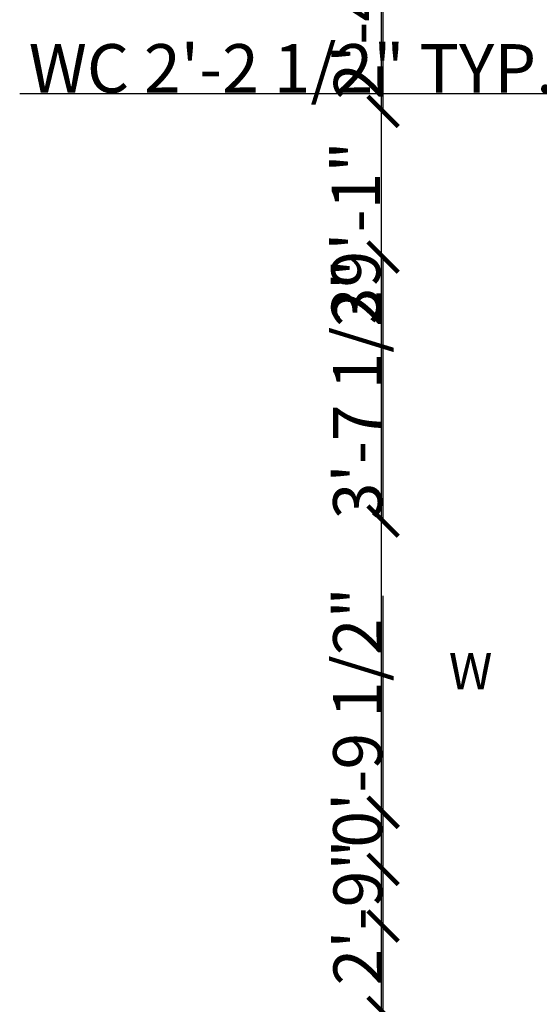
# Model space of a CAD drawing. Units: inches. Extents: x 2094 to 2639, y 1426 to 1997.
# Tile 2 of 8: x 2094 to 2180, y 1567 to 1730. Entities that reach past the tile are written whole.
import ezdxf

# ---------------------------------------------------------------- set-up
doc = ezdxf.new("R2010")
doc.units = ezdxf.units.IN
doc.layers.add('A-ANNO-DIMS', color=2, linetype='Continuous', lineweight=18)
doc.layers.add('A-ANNO-TEXT', color=7, linetype='Continuous', lineweight=18)
doc.styles.get("Standard").update_dxf_attribs({"font": 'arial.ttf'})
doc.dimstyles.get("Standard").update_dxf_attribs({"dimtxt": 8, "dimasz": 5, "dimexe": 0.18, "dimexo": 0.0625, "dimgap": 0.09, "dimtad": 1, "dimdec": 1, "dimzin": 0, "dimdsep": 46, "dimlunit": 4, "dimtxsty": 'Standard', "dimblk": 'ARCHTICK', "dimcen": 0.09, "dimse1": 1, "dimse2": 1, "dimadec": 0, "dimazin": 0, "dimtfac": 1, "dimtdec": 1, "dimtofl": 0, "dimtmove": 0, "dimatfit": 3, "dimfxl": 1, "dimtolj": 1, "dimtzin": 0, "dimarcsym": 0})

# ---------------------------------------------------------------- blocks, each defined once
blk = doc.blocks.new('_ArchTick')
at = {"color": 0, "linetype": 'ByBlock', "const_width": 0.15}
blk.add_lwpolyline([(-0.5, -0.5), (0.5, 0.5)], dxfattribs=at)
blk = doc.blocks.new('*D14')
at = {"layer": 'A-ANNO-DIMS', "color": 0, "lineweight": -2, "transparency": 16777216}
blk.add_line((2154, 1928.9), (2154, 1459.9), dxfattribs=at)
at = {"layer": 'Defpoints', "color": 0, "transparency": 16777216}
for p in [(2180.06, 1928.9), (2154, 1459.9), (2180.06, 1459.9)]:
    blk.add_point(p, dxfattribs=at)
at = {"layer": 'A-ANNO-DIMS', "color": 0, "lineweight": -2, "transparency": 16777216, "xscale": 5, "yscale": 5, "zscale": 5}
for p, rotation in [((2154, 1928.9), 90), ((2154, 1459.9), 270)]:
    blk.add_blockref('_ArchTick', p, dxfattribs=dict(at, rotation=rotation))
at = {"layer": 'A-ANNO-DIMS', "color": 0, "transparency": 16777216, "insert": (2149.82, 1694.4), "char_height": 8, "attachment_point": 5, "rotation": 90}
blk.add_mtext('\\A1;39\'-1"', dxfattribs=at)
blk = doc.blocks.new('*D39')
at = {"layer": 'A-ANNO-DIMS', "color": 0, "lineweight": -2, "transparency": 16777216}
for p, q in [((2189.06, 1717.27), (2094.42, 1717.27)), ((2215.64, 1717.27), (2189.06, 1717.27))]:
    blk.add_line(p, q, dxfattribs=at)
at = {"layer": 'Defpoints', "color": 0, "transparency": 16777216}
for p in [(2189.06, 1717.27), (2189.06, 1713.28), (2215.64, 1713.28)]:
    blk.add_point(p, dxfattribs=at)
at = {"layer": 'A-ANNO-DIMS', "color": 0, "lineweight": -2, "transparency": 16777216, "xscale": 5, "yscale": 5, "zscale": 5, "rotation": 180}
blk.add_blockref('_ArchTick', (2189.06, 1717.27), dxfattribs=at)
at = {"layer": 'A-ANNO-DIMS', "color": 0, "lineweight": -2, "transparency": 16777216, "xscale": 5, "yscale": 5, "zscale": 5}
blk.add_blockref('_ArchTick', (2215.64, 1717.27), dxfattribs=at)
at = {"layer": 'A-ANNO-DIMS', "color": 0, "transparency": 16777216, "insert": (2139.24, 1721.49), "char_height": 8, "attachment_point": 5}
blk.add_mtext('\\A1;WC 2\'-2 1/2" TYP.', dxfattribs=at)
blk = doc.blocks.new('*D56')
at = {"layer": 'A-ANNO-DIMS', "color": 0, "lineweight": -2, "transparency": 16777216}
blk.add_line((2154.31, 1565.9), (2154.31, 1598.9), dxfattribs=at)
at = {"layer": 'Defpoints', "color": 0, "transparency": 16777216}
for p in [(2154.31, 1598.9), (2180.06, 1598.9), (2189.06, 1565.9)]:
    blk.add_point(p, dxfattribs=at)
at = {"layer": 'A-ANNO-DIMS', "color": 0, "lineweight": -2, "transparency": 16777216, "xscale": 5, "yscale": 5, "zscale": 5}
for p, rotation in [((2154.31, 1598.9), 90), ((2154.31, 1565.9), 270)]:
    blk.add_blockref('_ArchTick', p, dxfattribs=dict(at, rotation=rotation))
at = {"layer": 'A-ANNO-DIMS', "color": 0, "transparency": 16777216, "insert": (2150.13, 1582.4), "char_height": 8, "attachment_point": 5, "rotation": 90}
blk.add_mtext('\\A1;2\'-9"', dxfattribs=at)
blk = doc.blocks.new('*D57')
at = {"layer": 'A-ANNO-DIMS', "color": 0, "lineweight": -2, "transparency": 16777216}
blk.add_line((2154.31, 1646.9), (2154.31, 1690.4), dxfattribs=at)
at = {"layer": 'Defpoints', "color": 0, "transparency": 16777216}
for p in [(2154.31, 1690.4), (2180.06, 1690.4), (2180.06, 1646.9)]:
    blk.add_point(p, dxfattribs=at)
at = {"layer": 'A-ANNO-DIMS', "color": 0, "lineweight": -2, "transparency": 16777216, "xscale": 5, "yscale": 5, "zscale": 5}
for p, rotation in [((2154.31, 1690.4), 90), ((2154.31, 1646.9), 270)]:
    blk.add_blockref('_ArchTick', p, dxfattribs=dict(at, rotation=rotation))
at = {"layer": 'A-ANNO-DIMS', "color": 0, "transparency": 16777216, "insert": (2150.08, 1668.65), "char_height": 8, "attachment_point": 5, "rotation": 90}
blk.add_mtext('\\A1;3\'-7 1/2"', dxfattribs=at)
blk = doc.blocks.new('*D58')
at = {"layer": 'A-ANNO-DIMS', "color": 0, "lineweight": -2, "transparency": 16777216}
blk.add_line((2154.31, 1714.4), (2154.31, 1742.37), dxfattribs=at)
at = {"layer": 'Defpoints', "color": 0, "transparency": 16777216}
for p in [(2154.31, 1742.37), (2180.06, 1742.37), (2180.06, 1714.4)]:
    blk.add_point(p, dxfattribs=at)
at = {"layer": 'A-ANNO-DIMS', "color": 0, "lineweight": -2, "transparency": 16777216, "xscale": 5, "yscale": 5, "zscale": 5}
for p, rotation in [((2154.31, 1742.37), 90), ((2154.31, 1714.4), 270)]:
    blk.add_blockref('_ArchTick', p, dxfattribs=dict(at, rotation=rotation))
at = {"layer": 'A-ANNO-DIMS', "color": 0, "transparency": 16777216, "insert": (2150.2, 1728.38), "char_height": 8, "attachment_point": 5, "rotation": 90}
blk.add_mtext('\\A1;2\'-4"', dxfattribs=at)
blk = doc.blocks.new('*D82')
at = {"layer": 'A-ANNO-DIMS', "color": 0, "lineweight": -2, "transparency": 16777216}
for p, q in [((2154.31, 1589.48), (2154.31, 1634.57)), ((2154.31, 1580.13), (2154.31, 1589.48))]:
    blk.add_line(p, q, dxfattribs=at)
at = {"layer": 'Defpoints', "color": 0, "transparency": 16777216}
for p in [(2154.31, 1589.48), (2249.13, 1589.48), (2249.13, 1580.13)]:
    blk.add_point(p, dxfattribs=at)
at = {"layer": 'A-ANNO-DIMS', "color": 0, "lineweight": -2, "transparency": 16777216, "xscale": 5, "yscale": 5, "zscale": 5}
for p, rotation in [((2154.31, 1589.48), 90), ((2154.31, 1580.13), 270)]:
    blk.add_blockref('_ArchTick', p, dxfattribs=dict(at, rotation=rotation))
at = {"layer": 'A-ANNO-DIMS', "color": 0, "transparency": 16777216, "insert": (2150.08, 1614.53), "char_height": 8, "attachment_point": 5, "rotation": 90}
blk.add_mtext('\\A1;0\'-9 1/2"', dxfattribs=at)

msp = doc.modelspace()

# ---------------------------------------------------------------- texts
at = {"layer": 'A-ANNO-TEXT'}
msp.add_text('W', height=6, dxfattribs=at).set_placement((2165.14, 1619.15))

# ---------------------------------------------------------------- dimensions: what is measured, and where the dimension line sits
at = {"layer": 'A-ANNO-DIMS'}
for base, p1, p2, override, picture, middle in [((2154, 1459.9), (2180.06, 1928.9), (2180.06, 1459.9), {"dimclrd": 0, "dimclre": 0, "dimclrt": 0}, '*D14', (2149.82, 1694.4)), ((2154.31, 1742.37), (2180.06, 1714.4), (2180.06, 1742.37), {"dimdec": 1, "dimlfac": 1, "dimrnd": 0, "dimzin": 1, "dimdsep": 46, "dimlunit": 4, "dimfrac": 2}, '*D58', (2150.2, 1728.38)), ((2154.31, 1690.4), (2180.06, 1646.9), (2180.06, 1690.4), {"dimdec": 1, "dimlfac": 1, "dimrnd": 0, "dimzin": 1, "dimdsep": 46, "dimlunit": 4, "dimfrac": 2}, '*D57', (2150.08, 1668.65)), ((2154.3063, 1589.4845), (2249.1311, 1580.1261), (2249.1311, 1589.4845), {"dimdec": 1, "dimlfac": 1, "dimrnd": 0, "dimzin": 1, "dimdsep": 46, "dimlunit": 4, "dimfrac": 2}, '*D82', (2150.0799, 1614.5281)), ((2154.31, 1598.9), (2189.06, 1565.9), (2180.06, 1598.9), {"dimdec": 1, "dimlfac": 1, "dimrnd": 0, "dimzin": 1, "dimdsep": 46, "dimlunit": 4, "dimfrac": 2}, '*D56', (2150.13, 1582.4))]:
    dim = msp.add_linear_dim(base=base, p1=p1, p2=p2, angle=90, dimstyle='Standard', override=override, dxfattribs=at)
    dim.commit()
    dim.dimension.update_dxf_attribs({"geometry": picture, "text_midpoint": middle})
dim = msp.add_linear_dim(base=(2189.06, 1717.27), p1=(2215.64, 1713.28), p2=(2189.06, 1713.28), angle=180, text='WC <> TYP.', dimstyle='Standard', override={"dimdec": 1, "dimlfac": 1, "dimrnd": 0, "dimzin": 1, "dimdsep": 46, "dimlunit": 4, "dimfrac": 2}, dxfattribs=at)
dim.commit()
dim.dimension.update_dxf_attribs({"geometry": '*D39', "text_midpoint": (2139.24, 1721.49)})

doc.saveas('drawing.dxf')
